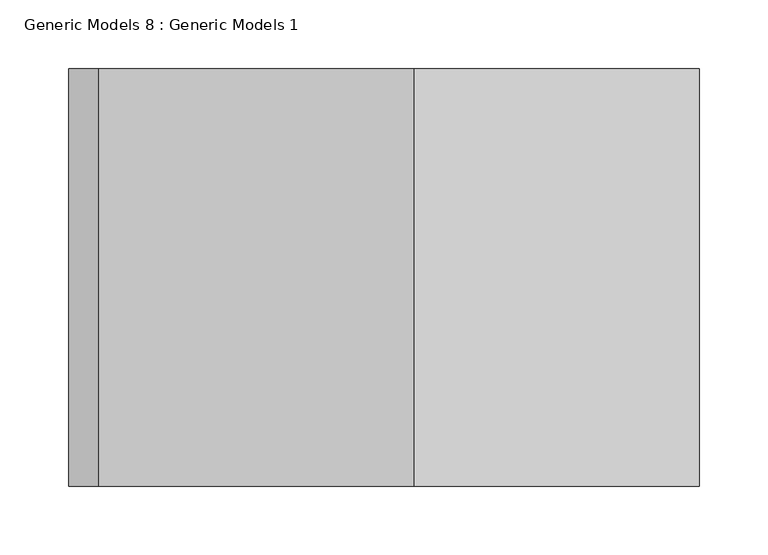
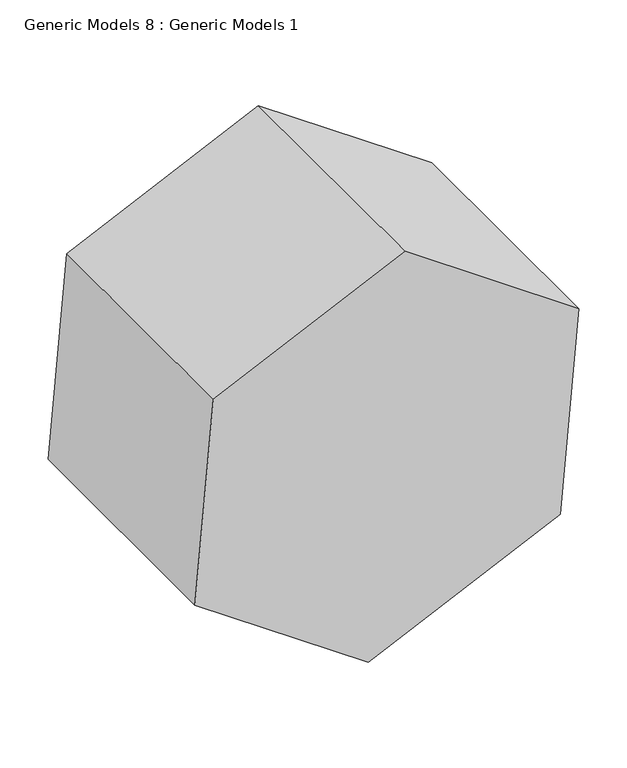
"""IFC4 building model written with IfcOpenShell, lengths in millimetres: proxy geometry, Generic Models 8 : Generic Models 1."""

from ifc_helpers import new_model, si_unit, frame, origin, place, context, project, spatial, polyline, outline, extrude, source, transform, mapped, element, save


def generic_models_8_generic_models_1_e8626bb7(model_context):
    return source(origin(), model_context, "Body", "SweptSolid", [
        extrude(outline(polyline([(833.1013393, 809.2920945), (978.7897542, 601.2274753), (871.4447157, 371.0252974), (618.4112624, 348.8877387), (472.7228475, 556.952358), (580.067886, 787.1545359), (833.1013393, 809.2920945)])), frame((0.0, -10720.3372434, 0.0), z_axis=(0.0, 1.0, 0.0), x_axis=(0.0, 0.0, 1.0)), (0.0, 0.0, 1.0), 304.8),
    ])


if __name__ == "__main__":
    model = new_model("IFC4")
    model_context = context("Model", 3, world=origin())
    ifc_project = project(units=[si_unit("LENGTHUNIT", "METRE", prefix="MILLI")], contexts=[model_context])
    site = spatial("IfcSite", under=ifc_project)
    building = spatial("IfcBuilding", under=site)
    placement = place(None, origin())
    generic_models_8_generic_models_1_shape = generic_models_8_generic_models_1_e8626bb7(model_context)
    element("IfcBuildingElementProxy", 1, Name="Generic Models 8 : Generic Models 1", ObjectType="Generic Models 8 : Generic Models 1", at=placement, inside=building, context=model_context, shape_type="MappedRepresentation", body=[
        mapped(generic_models_8_generic_models_1_shape, transform((0.0, 0.0, 0.0), x_axis=(1.0, 0.0, 0.0), y_axis=(0.0, 1.0, 0.0), z_axis=(0.0, 0.0, 1.0))),
    ])
    save(model, "model.ifc")

# Revit data of these elements
# Element 1 (IfcBuildingElementProxy, "Generic Models 8 : Generic Models 1")
#   Materials on its faces: "Carpet (1)"
# Materials
#   "Carpet (1)": class "Carpet", colour RGB 124 80 67, transparency 0, Description = "Interior finish", Cost = 0
